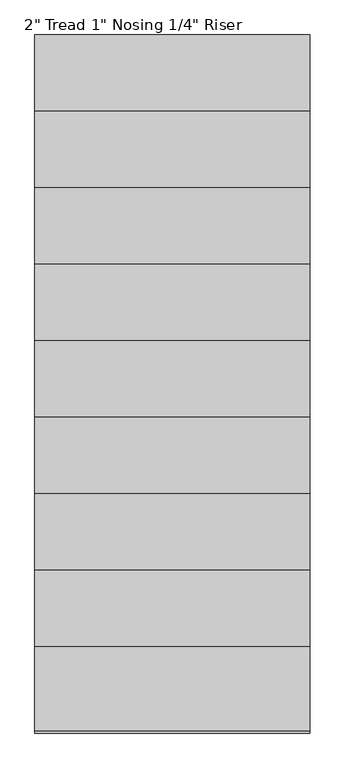
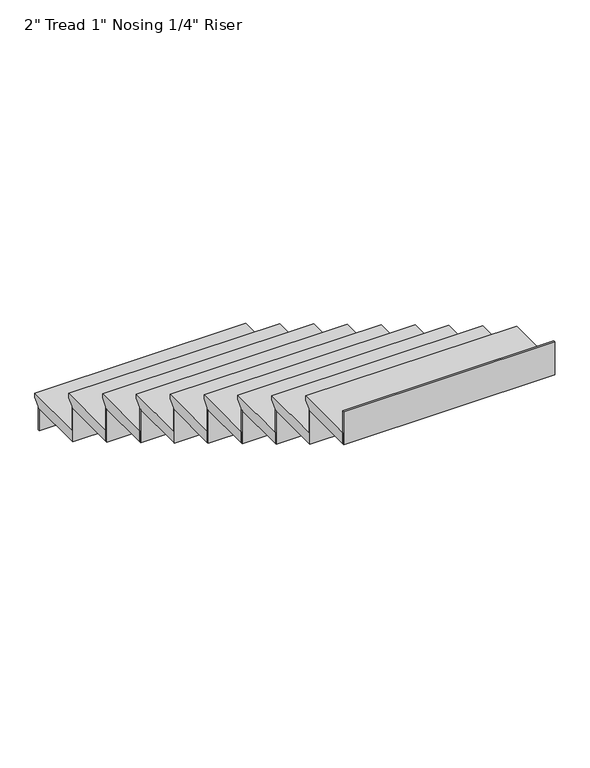
"""IFC4 building model written with IfcOpenShell, lengths in millimetres: stair flight geometry."""

from ifc_helpers import new_model, si_unit, origin, place, context, project, spatial, faceted_brep, source, transform, mapped, element, save


def stair_flight_f1905681(model_context):
    return source(origin(), model_context, "Body", "Brep", [
        faceted_brep([(-4315.1137331, -4241.0593836, 3333.75), (-4315.1137331, -4241.0593836, 3352.8), (-3400.7137331, -4241.0593836, 3352.8), (-3400.7137331, -4241.0593836, 3333.75), (-4315.1137331, -4266.4593836, 3308.35), (-3400.7137331, -4266.4593836, 3308.35), (-4315.1137331, -4520.4593836, 3352.8), (-3400.7137331, -4520.4593836, 3352.8), (-3400.7137331, -4266.4593836, 3302.0), (-3400.7137331, -4520.4593836, 3302.0), (-4315.1137331, -4520.4593836, 3302.0), (-4315.1137331, -4266.4593836, 3302.0)], [[[0, 1, 2, 3]], [[4, 0, 3, 5]], [[2, 1, 6, 7]], [[8, 9, 10, 11]], [[2, 7, 9, 8, 5, 3]], [[8, 11, 4, 5]], [[6, 1, 0, 4, 11, 10]], [[7, 6, 10, 9]]]),
        faceted_brep([(-4315.1137331, -4266.4593836, 3302.0), (-4315.1137331, -4266.4593836, 3200.4), (-4315.1137331, -4272.8093836, 3200.4), (-4315.1137331, -4272.8093836, 3302.0), (-3400.7137331, -4266.4593836, 3302.0), (-3400.7137331, -4272.8093836, 3302.0), (-3400.7137331, -4272.8093836, 3200.4), (-3400.7137331, -4266.4593836, 3200.4)], [[[0, 1, 2, 3]], [[4, 5, 6, 7]], [[1, 0, 4, 7]], [[2, 1, 7, 6]], [[3, 2, 6, 5]], [[0, 3, 5, 4]]]),
        faceted_brep([(-4315.1137331, -4520.4593836, 3454.4), (-4315.1137331, -4520.4593836, 3302.0), (-4315.1137331, -4526.8093836, 3302.0), (-4315.1137331, -4526.8093836, 3454.4), (-3400.7137331, -4520.4593836, 3454.4), (-3400.7137331, -4526.8093836, 3454.4), (-3400.7137331, -4526.8093836, 3302.0), (-3400.7137331, -4520.4593836, 3302.0)], [[[0, 1, 2, 3]], [[4, 5, 6, 7]], [[1, 0, 4, 7]], [[2, 1, 7, 6]], [[3, 2, 6, 5]], [[0, 3, 5, 4]]]),
        faceted_brep([(-3400.7137331, -4495.0593836, 3505.2), (-4315.1137331, -4495.0593836, 3505.2), (-4315.1137331, -4774.4593836, 3505.2), (-3400.7137331, -4774.4593836, 3505.2), (-3400.7137331, -4520.4593836, 3454.4), (-3400.7137331, -4774.4593836, 3454.4), (-4315.1137331, -4774.4593836, 3454.4), (-4315.1137331, -4520.4593836, 3454.4), (-3400.7137331, -4520.4593836, 3460.75), (-3400.7137331, -4495.0593836, 3486.15), (-4315.1137331, -4520.4593836, 3460.75), (-4315.1137331, -4495.0593836, 3486.15)], [[[0, 1, 2, 3]], [[4, 5, 6, 7]], [[0, 3, 5, 4, 8, 9]], [[4, 7, 10, 8]], [[2, 1, 11, 10, 7, 6]], [[3, 2, 6, 5]], [[11, 1, 0, 9]], [[10, 11, 9, 8]]]),
        faceted_brep([(-4315.1137331, -4774.4593836, 3606.8), (-4315.1137331, -4774.4593836, 3454.4), (-4315.1137331, -4780.8093836, 3454.4), (-4315.1137331, -4780.8093836, 3606.8), (-3400.7137331, -4774.4593836, 3606.8), (-3400.7137331, -4780.8093836, 3606.8), (-3400.7137331, -4780.8093836, 3454.4), (-3400.7137331, -4774.4593836, 3454.4)], [[[0, 1, 2, 3]], [[4, 5, 6, 7]], [[1, 0, 4, 7]], [[2, 1, 7, 6]], [[3, 2, 6, 5]], [[0, 3, 5, 4]]]),
        faceted_brep([(-3400.7137331, -4749.0593836, 3657.6), (-4315.1137331, -4749.0593836, 3657.6), (-4315.1137331, -5028.4593836, 3657.6), (-3400.7137331, -5028.4593836, 3657.6), (-3400.7137331, -4774.4593836, 3606.8), (-3400.7137331, -5028.4593836, 3606.8), (-4315.1137331, -5028.4593836, 3606.8), (-4315.1137331, -4774.4593836, 3606.8), (-3400.7137331, -4774.4593836, 3613.15), (-3400.7137331, -4749.0593836, 3638.55), (-4315.1137331, -4774.4593836, 3613.15), (-4315.1137331, -4749.0593836, 3638.55)], [[[0, 1, 2, 3]], [[4, 5, 6, 7]], [[0, 3, 5, 4, 8, 9]], [[4, 7, 10, 8]], [[2, 1, 11, 10, 7, 6]], [[3, 2, 6, 5]], [[11, 1, 0, 9]], [[10, 11, 9, 8]]]),
        faceted_brep([(-4315.1137331, -5028.4593836, 3759.2), (-4315.1137331, -5028.4593836, 3606.8), (-4315.1137331, -5034.8093836, 3606.8), (-4315.1137331, -5034.8093836, 3759.2), (-3400.7137331, -5028.4593836, 3759.2), (-3400.7137331, -5034.8093836, 3759.2), (-3400.7137331, -5034.8093836, 3606.8), (-3400.7137331, -5028.4593836, 3606.8)], [[[0, 1, 2, 3]], [[4, 5, 6, 7]], [[1, 0, 4, 7]], [[2, 1, 7, 6]], [[3, 2, 6, 5]], [[0, 3, 5, 4]]]),
        faceted_brep([(-3400.7137331, -5003.0593836, 3810.0), (-4315.1137331, -5003.0593836, 3810.0), (-4315.1137331, -5282.4593836, 3810.0), (-3400.7137331, -5282.4593836, 3810.0), (-3400.7137331, -5028.4593836, 3759.2), (-3400.7137331, -5282.4593836, 3759.2), (-4315.1137331, -5282.4593836, 3759.2), (-4315.1137331, -5028.4593836, 3759.2), (-3400.7137331, -5028.4593836, 3765.55), (-3400.7137331, -5003.0593836, 3790.95), (-4315.1137331, -5028.4593836, 3765.55), (-4315.1137331, -5003.0593836, 3790.95)], [[[0, 1, 2, 3]], [[4, 5, 6, 7]], [[0, 3, 5, 4, 8, 9]], [[4, 7, 10, 8]], [[2, 1, 11, 10, 7, 6]], [[3, 2, 6, 5]], [[11, 1, 0, 9]], [[10, 11, 9, 8]]]),
        faceted_brep([(-4315.1137331, -5282.4593836, 3911.6), (-4315.1137331, -5282.4593836, 3759.2), (-4315.1137331, -5288.8093836, 3759.2), (-4315.1137331, -5288.8093836, 3911.6), (-3400.7137331, -5282.4593836, 3911.6), (-3400.7137331, -5288.8093836, 3911.6), (-3400.7137331, -5288.8093836, 3759.2), (-3400.7137331, -5282.4593836, 3759.2)], [[[0, 1, 2, 3]], [[4, 5, 6, 7]], [[1, 0, 4, 7]], [[2, 1, 7, 6]], [[3, 2, 6, 5]], [[0, 3, 5, 4]]]),
        faceted_brep([(-3400.7137331, -5257.0593836, 3962.4), (-4315.1137331, -5257.0593836, 3962.4), (-4315.1137331, -5536.4593836, 3962.4), (-3400.7137331, -5536.4593836, 3962.4), (-3400.7137331, -5282.4593836, 3911.6), (-3400.7137331, -5536.4593836, 3911.6), (-4315.1137331, -5536.4593836, 3911.6), (-4315.1137331, -5282.4593836, 3911.6), (-3400.7137331, -5282.4593836, 3917.95), (-3400.7137331, -5257.0593836, 3943.35), (-4315.1137331, -5282.4593836, 3917.95), (-4315.1137331, -5257.0593836, 3943.35)], [[[0, 1, 2, 3]], [[4, 5, 6, 7]], [[0, 3, 5, 4, 8, 9]], [[4, 7, 10, 8]], [[2, 1, 11, 10, 7, 6]], [[3, 2, 6, 5]], [[11, 1, 0, 9]], [[10, 11, 9, 8]]]),
        faceted_brep([(-4315.1137331, -5536.4593836, 4064.0), (-4315.1137331, -5536.4593836, 3911.6), (-4315.1137331, -5542.8093836, 3911.6), (-4315.1137331, -5542.8093836, 4064.0), (-3400.7137331, -5536.4593836, 4064.0), (-3400.7137331, -5542.8093836, 4064.0), (-3400.7137331, -5542.8093836, 3911.6), (-3400.7137331, -5536.4593836, 3911.6)], [[[0, 1, 2, 3]], [[4, 5, 6, 7]], [[1, 0, 4, 7]], [[2, 1, 7, 6]], [[3, 2, 6, 5]], [[0, 3, 5, 4]]]),
        faceted_brep([(-3400.7137331, -5511.0593836, 4114.8), (-4315.1137331, -5511.0593836, 4114.8), (-4315.1137331, -5790.4593836, 4114.8), (-3400.7137331, -5790.4593836, 4114.8), (-3400.7137331, -5536.4593836, 4064.0), (-3400.7137331, -5790.4593836, 4064.0), (-4315.1137331, -5790.4593836, 4064.0), (-4315.1137331, -5536.4593836, 4064.0), (-3400.7137331, -5536.4593836, 4070.35), (-3400.7137331, -5511.0593836, 4095.75), (-4315.1137331, -5536.4593836, 4070.35), (-4315.1137331, -5511.0593836, 4095.75)], [[[0, 1, 2, 3]], [[4, 5, 6, 7]], [[0, 3, 5, 4, 8, 9]], [[4, 7, 10, 8]], [[2, 1, 11, 10, 7, 6]], [[3, 2, 6, 5]], [[11, 1, 0, 9]], [[10, 11, 9, 8]]]),
        faceted_brep([(-4315.1137331, -5790.4593836, 4216.4), (-4315.1137331, -5790.4593836, 4064.0), (-4315.1137331, -5796.8093836, 4064.0), (-4315.1137331, -5796.8093836, 4216.4), (-3400.7137331, -5790.4593836, 4216.4), (-3400.7137331, -5796.8093836, 4216.4), (-3400.7137331, -5796.8093836, 4064.0), (-3400.7137331, -5790.4593836, 4064.0)], [[[0, 1, 2, 3]], [[4, 5, 6, 7]], [[1, 0, 4, 7]], [[2, 1, 7, 6]], [[3, 2, 6, 5]], [[0, 3, 5, 4]]]),
        faceted_brep([(-3400.7137331, -5765.0593836, 4267.2), (-4315.1137331, -5765.0593836, 4267.2), (-4315.1137331, -6044.4593836, 4267.2), (-3400.7137331, -6044.4593836, 4267.2), (-3400.7137331, -5790.4593836, 4216.4), (-3400.7137331, -6044.4593836, 4216.4), (-4315.1137331, -6044.4593836, 4216.4), (-4315.1137331, -5790.4593836, 4216.4), (-3400.7137331, -5790.4593836, 4222.75), (-3400.7137331, -5765.0593836, 4248.15), (-4315.1137331, -5790.4593836, 4222.75), (-4315.1137331, -5765.0593836, 4248.15)], [[[0, 1, 2, 3]], [[4, 5, 6, 7]], [[0, 3, 5, 4, 8, 9]], [[4, 7, 10, 8]], [[2, 1, 11, 10, 7, 6]], [[3, 2, 6, 5]], [[11, 1, 0, 9]], [[10, 11, 9, 8]]]),
        faceted_brep([(-4315.1137331, -6044.4593836, 4368.8), (-4315.1137331, -6044.4593836, 4216.4), (-4315.1137331, -6050.8093836, 4216.4), (-4315.1137331, -6050.8093836, 4368.8), (-3400.7137331, -6044.4593836, 4368.8), (-3400.7137331, -6050.8093836, 4368.8), (-3400.7137331, -6050.8093836, 4216.4), (-3400.7137331, -6044.4593836, 4216.4)], [[[0, 1, 2, 3]], [[4, 5, 6, 7]], [[1, 0, 4, 7]], [[2, 1, 7, 6]], [[3, 2, 6, 5]], [[0, 3, 5, 4]]]),
        faceted_brep([(-3400.7137331, -6019.0593836, 4419.6), (-4315.1137331, -6019.0593836, 4419.6), (-4315.1137331, -6298.4593836, 4419.6), (-3400.7137331, -6298.4593836, 4419.6), (-3400.7137331, -6044.4593836, 4368.8), (-3400.7137331, -6298.4593836, 4368.8), (-4315.1137331, -6298.4593836, 4368.8), (-4315.1137331, -6044.4593836, 4368.8), (-3400.7137331, -6044.4593836, 4375.15), (-3400.7137331, -6019.0593836, 4400.55), (-4315.1137331, -6044.4593836, 4375.15), (-4315.1137331, -6019.0593836, 4400.55)], [[[0, 1, 2, 3]], [[4, 5, 6, 7]], [[0, 3, 5, 4, 8, 9]], [[4, 7, 10, 8]], [[2, 1, 11, 10, 7, 6]], [[3, 2, 6, 5]], [[11, 1, 0, 9]], [[10, 11, 9, 8]]]),
        faceted_brep([(-4315.1137331, -6552.4593836, 4673.6), (-4315.1137331, -6552.4593836, 4521.2), (-4315.1137331, -6558.8093836, 4521.2), (-4315.1137331, -6558.8093836, 4673.6), (-3400.7137331, -6552.4593836, 4673.6), (-3400.7137331, -6558.8093836, 4673.6), (-3400.7137331, -6558.8093836, 4521.2), (-3400.7137331, -6552.4593836, 4521.2)], [[[0, 1, 2, 3]], [[4, 5, 6, 7]], [[1, 0, 4, 7]], [[2, 1, 7, 6]], [[3, 2, 6, 5]], [[0, 3, 5, 4]]]),
        faceted_brep([(-4315.1137331, -6298.4593836, 4521.2), (-4315.1137331, -6298.4593836, 4368.8), (-4315.1137331, -6304.8093836, 4368.8), (-4315.1137331, -6304.8093836, 4521.2), (-3400.7137331, -6298.4593836, 4521.2), (-3400.7137331, -6304.8093836, 4521.2), (-3400.7137331, -6304.8093836, 4368.8), (-3400.7137331, -6298.4593836, 4368.8)], [[[0, 1, 2, 3]], [[4, 5, 6, 7]], [[1, 0, 4, 7]], [[2, 1, 7, 6]], [[3, 2, 6, 5]], [[0, 3, 5, 4]]]),
        faceted_brep([(-3400.7137331, -6552.4593836, 4572.0), (-3400.7137331, -6527.0593836, 4572.0), (-3400.7137331, -6273.0593836, 4572.0), (-4315.1137331, -6273.0593836, 4572.0), (-4315.1137331, -6552.4593836, 4572.0), (-3400.7137331, -6527.0593836, 4521.2), (-3400.7137331, -6552.4593836, 4521.2), (-4315.1137331, -6552.4593836, 4521.2), (-4315.1137331, -6298.4593836, 4521.2), (-3400.7137331, -6298.4593836, 4521.2), (-3400.7137331, -6298.4593836, 4527.55), (-3400.7137331, -6273.0593836, 4552.95), (-4315.1137331, -6298.4593836, 4527.55), (-4315.1137331, -6273.0593836, 4552.95)], [[[0, 1, 2, 3, 4]], [[5, 6, 7, 8, 9]], [[1, 0, 6, 5]], [[2, 1, 5, 9, 10, 11]], [[9, 8, 12, 10]], [[4, 3, 13, 12, 8, 7]], [[0, 4, 7, 6]], [[13, 3, 2, 11]], [[12, 13, 11, 10]]]),
    ])


if __name__ == "__main__":
    model = new_model("IFC4")
    model_context = context("Model", 3, world=origin())
    ifc_project = project(units=[si_unit("LENGTHUNIT", "METRE", prefix="MILLI")], contexts=[model_context])
    site = spatial("IfcSite", under=ifc_project)
    building = spatial("IfcBuilding", under=site)
    placement = place(None, origin())
    stair_flight_shape = stair_flight_f1905681(model_context)
    element("IfcStairFlight", 1, ObjectType="2\" Tread 1\" Nosing 1/4\" Riser", at=placement, inside=building, context=model_context, shape_type="MappedRepresentation", body=[
        mapped(stair_flight_shape, transform((0.0, 0.0, 0.0), x_axis=(1.0, 0.0, 0.0), y_axis=(0.0, 1.0, 0.0), z_axis=(0.0, 0.0, 1.0))),
    ])
    save(model, "model.ifc")
